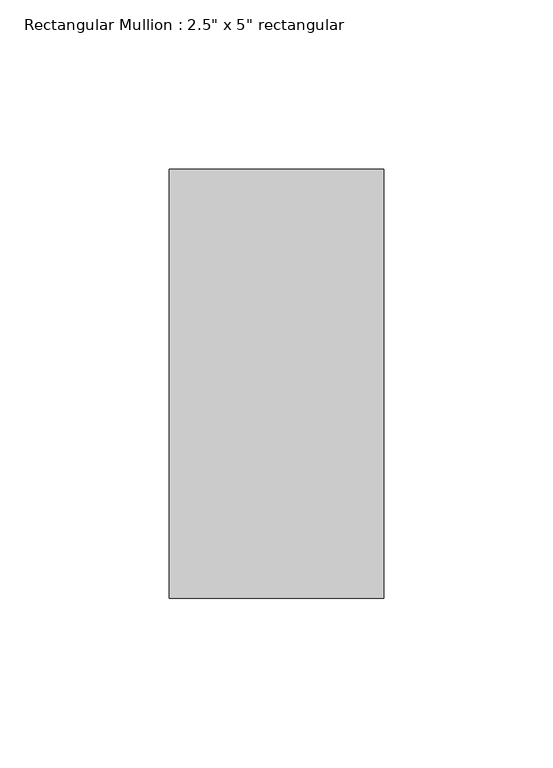
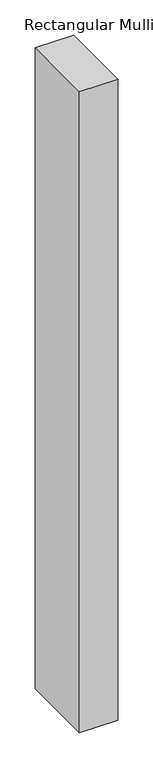
"""IFC4 building model written with IfcOpenShell, lengths in millimetres: member geometry."""

from ifc_helpers import new_model, si_unit, frame, origin, place, context, project, spatial, polyline, outline, extrude, source, transform, mapped, element, save


def member_02c0e4c4(model_context):
    return source(origin(), model_context, "Body", "SweptSolid", [
        extrude(outline(polyline([(0.0, 63.5), (0.0, -63.5), (-63.5, -63.5), (-63.5, 63.5), (0.0, 63.5)])), frame((0.0, 0.0, -1117.6), z_axis=(0.0, 0.0, 1.0), x_axis=(1.0, 0.0, 0.0)), (0.0, 0.0, 1.0), 1117.6),
    ])


if __name__ == "__main__":
    model = new_model("IFC4")
    model_context = context("Model", 3, world=origin())
    ifc_project = project(units=[si_unit("LENGTHUNIT", "METRE", prefix="MILLI")], contexts=[model_context])
    site = spatial("IfcSite", under=ifc_project)
    building = spatial("IfcBuilding", under=site)
    placement = place(None, origin())
    member_shape = member_02c0e4c4(model_context)
    element("IfcMember", 1, ObjectType="Rectangular Mullion : 2.5\" x 5\" rectangular", at=placement, inside=building, context=model_context, shape_type="MappedRepresentation", body=[
        mapped(member_shape, transform((0.0, 0.0, 0.0), x_axis=(1.0, 0.0, 0.0), y_axis=(0.0, 1.0, 0.0), z_axis=(0.0, 0.0, 1.0))),
    ])
    save(model, "model.ifc")

# Revit data of these elements
# Type "Rectangular Mullion : 2.5\" x 5\" rectangular"
#   built-in parameter 1007304 = 0.416667 (stored number, unit not read)
#   built-in parameter 1007301 = 0.104167 (stored number, unit not read)
#   built-in parameter 1007300 = 0.104167 (stored number, unit not read)
# Element 1 (IfcMember, "Rectangular Mullion : 2.5\" x 5\" rectangular")
#   Materials on its faces: "Aluminum"
# Materials
#   "Aluminum": class "Metal", colour RGB 247 247 247, transparency 0, Description = "Aluminum 6061", Cost = 0
